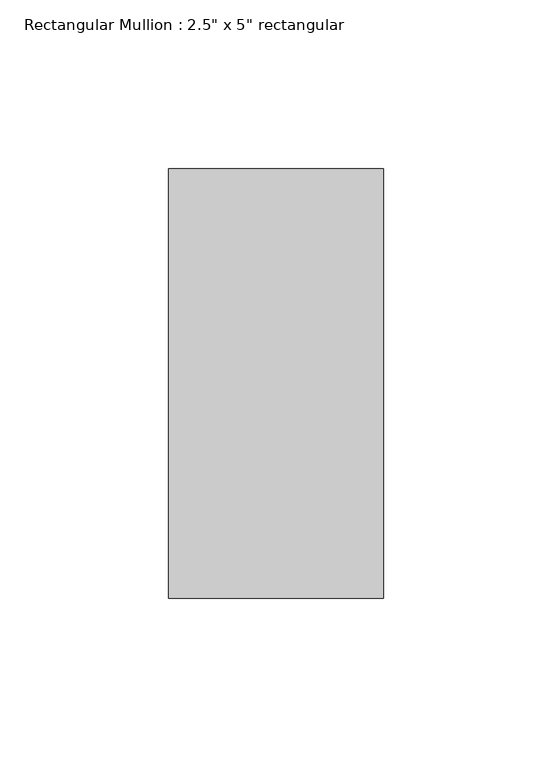
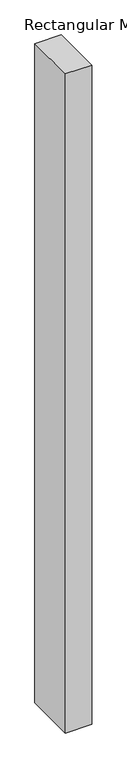
"""IFC4 building model written with IfcOpenShell, lengths in millimetres: member geometry."""

from ifc_helpers import new_model, si_unit, frame, origin, place, context, project, spatial, polyline, outline, extrude, source, transform, mapped, element, save


def member_062c1ce8(model_context):
    return source(origin(), model_context, "Body", "SweptSolid", [
        extrude(outline(polyline([(0.0, 63.5), (0.0, -63.5), (-63.5, -63.5), (-63.5, 63.5), (0.0, 63.5)])), frame((0.0, 0.0, -1676.4), z_axis=(0.0, 0.0, 1.0), x_axis=(1.0, 0.0, 0.0)), (0.0, 0.0, 1.0), 1676.4),
    ])


if __name__ == "__main__":
    model = new_model("IFC4")
    model_context = context("Model", 3, world=origin())
    ifc_project = project(units=[si_unit("LENGTHUNIT", "METRE", prefix="MILLI")], contexts=[model_context])
    site = spatial("IfcSite", under=ifc_project)
    building = spatial("IfcBuilding", under=site)
    placement = place(None, origin())
    member_shape = member_062c1ce8(model_context)
    element("IfcMember", 1, ObjectType="Rectangular Mullion : 2.5\" x 5\" rectangular", at=placement, inside=building, context=model_context, shape_type="MappedRepresentation", body=[
        mapped(member_shape, transform((0.0, 0.0, 0.0), x_axis=(1.0, 0.0, 0.0), y_axis=(0.0, 1.0, 0.0), z_axis=(0.0, 0.0, 1.0))),
    ])
    save(model, "model.ifc")

# Revit data of these elements
# Type "Rectangular Mullion : 2.5\" x 5\" rectangular"
#   built-in parameter 1007304 = 0.416667 (stored number, unit not read)
#   built-in parameter 1007301 = 0.104167 (stored number, unit not read)
#   built-in parameter 1007300 = 0.104167 (stored number, unit not read)
